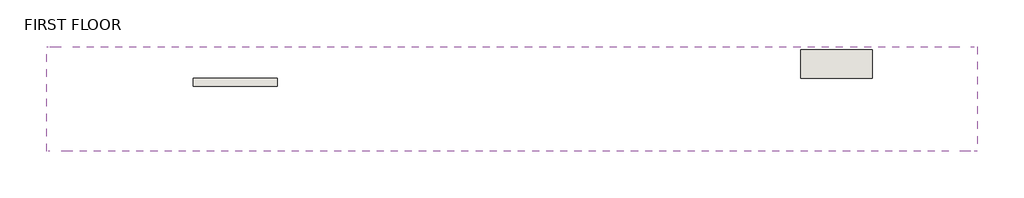
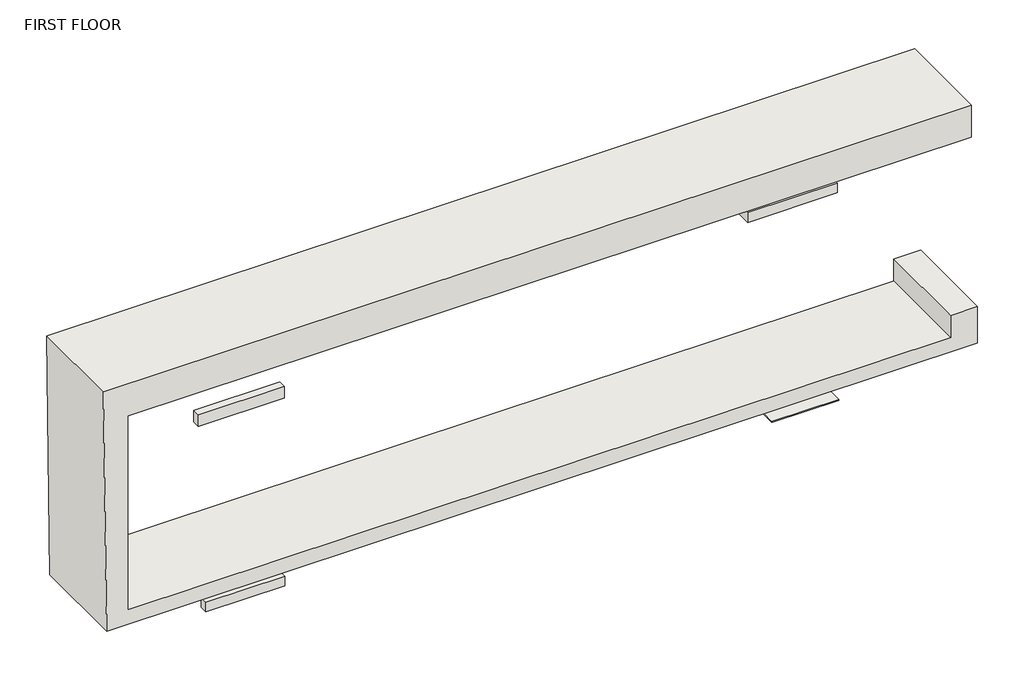
# One storey: 2 walls.
"""IFC4 building model written with IfcOpenShell, lengths in millimetres."""

from ifc_helpers import new_model, si_unit, origin, place, context, project, spatial, transform, mapped, element, save
from components import walls_2_walls_2_9d43e08d, walls_3_walls_3_d3df9a77

model = new_model("IFC4")

# Units and contexts
model_context = context("Model", 3, world=origin())
ifc_project = project(units=[si_unit("LENGTHUNIT", "METRE", prefix="MILLI")], contexts=[model_context])

# Site, building, storey
site = spatial("IfcSite", under=ifc_project)
building = spatial("IfcBuilding", under=site)
storey = spatial("IfcBuildingStorey", under=building, Name="FIRST FLOOR", Elevation=3048.0)

# Walls
placement = place(None, origin())
walls_2_walls_2_shape = walls_2_walls_2_9d43e08d(model_context)
element("IfcWall", 1, ObjectType="Walls 2 : Walls 2", at=placement, inside=storey, context=model_context, shape_type="MappedRepresentation", body=[
    mapped(walls_2_walls_2_shape, transform((0.0, 0.0, 0.0), x_axis=(1.0, 0.0, 0.0), y_axis=(0.0, 1.0, 0.0), z_axis=(0.0, 0.0, 1.0))),
])
walls_3_walls_3_shape = walls_3_walls_3_d3df9a77(model_context)
element("IfcWall", 2, ObjectType="Walls 3 : Walls 3", at=placement, inside=storey, context=model_context, shape_type="MappedRepresentation", body=[
    mapped(walls_3_walls_3_shape, transform((0.0, 0.0, 0.0), x_axis=(1.0, 0.0, 0.0), y_axis=(0.0, 1.0, 0.0), z_axis=(0.0, 0.0, 1.0))),
])

save(model, "model.ifc")

# Revit data of these elements
# Element 1 (IfcWall, "Walls 2 : Walls 2")
#   Phase Created = New Construction
#   Materials on its faces: "Default Wall"
# Element 2 (IfcWall, "Walls 3 : Walls 3")
#   Phase Created = New Construction
#   Materials on its faces: "Default Wall"
# Materials
#   "Default Wall": colour RGB 80 80 80, transparency 0
